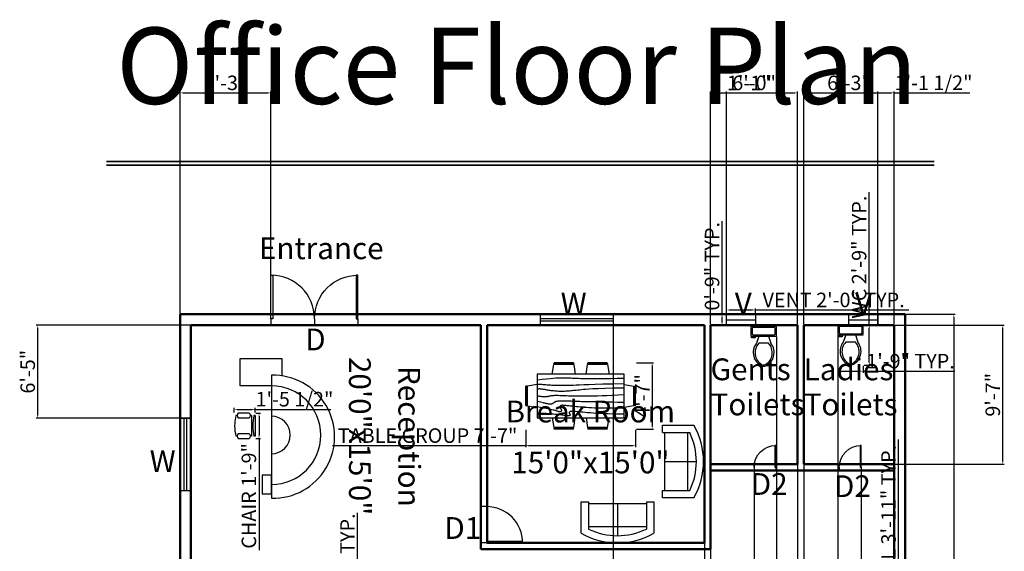
# Model space of a CAD drawing. Units: inches. Extents: x 1953 to 3378, y 1378 to 2530.
# Tile 4 of 5: x 1963 to 2778, y 2090 to 2530. Entities that reach past the tile are written whole.
import ezdxf

# ---------------------------------------------------------------- set-up
doc = ezdxf.new("R2010")
doc.units = ezdxf.units.IN
for name, color, linetype, lineweight in [('A-ANNO-DIMS', 2, 'Continuous', 18), ('A-ANNO-TEXT', 7, 'Continuous', 18), ('A-ANNO-TTLB', 7, 'Continuous', 35), ('A-AREA-IDEN', 4, 'Continuous', 18), ('A-DOOR', 4, 'Continuous', 25), ('A-FLOR-FIXT', 9, 'Continuous', 25), ('A-FURN', 50, 'Continuous', 25), ('wall', 7, 'Continuous', 50), ('windows', 180, 'Continuous', 25)]:
    doc.layers.add(name, color=color, linetype=linetype, lineweight=lineweight)
doc.styles.get("Standard").update_dxf_attribs({"font": 'arial.ttf'})
doc.dimstyles.new('ISO-25', dxfattribs={"dimtxt": 12, "dimasz": 2.5, "dimexe": 1.25, "dimexo": 0.625, "dimtad": 1, "dimdec": 1, "dimlunit": 4, "dimtxsty": 'Standard', "dimcen": 2.5, "dimadec": 0, "dimazin": 0, "dimtfac": 1, "dimtdec": 1, "dimtmove": 0, "dimatfit": 3, "dimfxl": 1, "dimarcsym": 0})

# ---------------------------------------------------------------- blocks, each defined once
blk = doc.blocks.new('*U7')
for p, q in [((0, 0), (0, -6)), ((-40, 0), (-40, -6))]:
    blk.add_line(p, q)
blk.add_lwpolyline([(0, 0), (0, 40), (-1.75, 40), (-1.75, 0)], close=True)
blk.add_arc((0, 0), 40, 90, 180)
blk = doc.blocks.new('*U2')
for p, q in [((0, 0), (0, -6)), ((40, 0), (40, -6))]:
    blk.add_line(p, q)
blk.add_lwpolyline([(0, 0), (0, 40), (1.75, 40), (1.75, 0)], close=True)
blk.add_arc((0, 0), 40, 0, 90)
blk = doc.blocks.new('Toilet - top')
for p, q in [((-8, -8.5), (-8, -8)), ((-7, -8), (-7, -9.5)), ((-4, -8), (-6, -14)), ((4, -8), (6, -14)), ((9.5, -6), (9.5, -2)), ((-10, -8.5), (-8, -8.5)), ((-10, -9.5), (-10, -8.5)), ((-7, -9.5), (-10, -9.5)), ((4, -14), (-4, -14))]:
    blk.add_line(p, q)
blk.add_lwpolyline([(10.5, -8), (10.5, 0), (-10.5, 0), (-10.5, -8)], close=True)
for points in [[(-9.5, -2), (-9.5, -6)], [(8.5, -1), (-8.5, -1)], [(-8.5, -7), (8.5, -7)]]:
    blk.add_lwpolyline(points)
for centre, radius, start, end in [((-8.62, -1.88), 0.884, 81.8699, 188.1301), ((-8.62, -6.12), 0.884, 171.8699, 278.1301), ((8.62, -1.88), 0.884, 351.8699, 98.1301), ((8.62, -6.12), 0.884, 261.8699, 8.1301), ((3.52, -21.58), 12.17, 141.46911, 247.97143), ((4.2, -21.82), 11.33, 136.36773, 238.94682), ((-3.52, -21.58), 12.17, 292.02843, 38.53071), ((-4.2, -21.82), 11.33, 301.05301, 43.63209), ((0, -27.88), 4, 245.73182, 294.26817), ((0, -29), 4, 254.86053, 285.13947)]:
    blk.add_arc(centre, radius, start, end)
blk = doc.blocks.new('Sofa - Roundback Loveseat 5 ft.')
for p, q in [((0, -32.44198), (0, -5.99998)), ((-24, -33.99998), (-24, -11.46958)), ((-23.9998, -13.38178), (23.99986, -13.38178)), ((24.00004, -33.99998), (24.00004, -11.46958)), ((-24, -32.44198), (24.00004, -32.44198))]:
    blk.add_line(p, q)
for points in [[(-24, -33.99998), (-30, -33.99998), (-30, -7.99998)], [(30.00004, -7.99998), (30.00004, -33.99998), (24.00004, -33.99998)]]:
    blk.add_lwpolyline(points)
for centre, radius, start, end in [((0, -60.24998), 60.24998, 60.13715, 119.8628), ((0, -61.38438), 55.38444, 64.32083, 115.6792)]:
    blk.add_arc(centre, radius, start, end)
blk = doc.blocks.new('Dining Set - 36 x 72 in.')
for p, q in [((-22.2343, 26.00059), (-23.4847, 17.99762)), ((-22.2304, 26), (-5.7608, 26)), ((-22, 27.5), (-22.1562, 26.50042)), ((-5.8416, 26.5), (-22.1534, 26.5)), ((-22, 27.5), (-6, 27.5)), ((-5.8437, 26.49966), (-6, 27.5)), ((-4.5152, 17.99762), (-5.7655, 25.99926)), ((5.7657, 26.00059), (4.5153, 17.99762)), ((5.7696, 26), (22.2392, 26)), ((6, 27.5), (5.8438, 26.50042)), ((22.1584, 26.5), (5.8466, 26.5)), ((6, 27.5), (22, 27.5)), ((22.1563, 26.49966), (22, 27.5)), ((23.4848, 17.99762), (22.2345, 25.99926)), ((36, 18), (-36, 18)), ((-36, 18), (-36, -18)), ((36, -18), (36, 18)), ((-45.5, 8), (-44.5004, 8.15617)), ((-44.5, -8.15843), (-44.5, 8.15338)), ((-44.0006, 8.23428), (-35.9976, 9.48474)), ((-44, 8.23041), (-44, -8.23915)), ((44.0006, 8.23428), (35.9976, 9.48474)), ((44, 8.23041), (44, -8.23915)), ((44.5, -8.15843), (44.5, 8.15338)), ((45.5, 8), (44.5005, 8.15617)), ((-45.5, 8), (-45.5, -8)), ((45.5, 8), (45.5, -8)), ((-44.4997, -8.15631), (-45.5, -8)), ((44.4997, -8.15631), (45.5, -8)), ((-35.9976, -9.48476), (-43.9993, -8.2345)), ((35.9976, -9.48476), (43.9993, -8.2345)), ((-36, -18), (36, -18)), ((-22.2343, -26.0006), (-23.4847, -17.99762)), ((-4.5152, -17.99762), (-5.7655, -25.99928)), ((5.7657, -26.0006), (4.5153, -17.99762)), ((23.4848, -17.99762), (22.2345, -25.99928)), ((-22.2304, -26), (-5.7608, -26)), ((-22, -27.5), (-22.1562, -26.50044)), ((-5.8416, -26.5), (-22.1534, -26.5)), ((-22, -27.5), (-6, -27.5)), ((-5.8437, -26.49967), (-6, -27.5)), ((5.7696, -26), (22.2392, -26)), ((6, -27.5), (5.8438, -26.50044)), ((22.1584, -26.5), (5.8466, -26.5)), ((6, -27.5), (22, -27.5)), ((22.1563, -26.49967), (22, -27.5))]:
    blk.add_line(p, q)
for points in [[(-36, 15), (-31.1772, 14.97754), (-26.8079, 14.91406), (-22.8538, 14.81543), (-19.276, 14.6875), (-16.0362, 14.53613), (-13.0957, 14.36718), (-10.4159, 14.18652), (-7.9583, 14), (-5.6904, 13.81315), (-3.6035, 13.63021), (-1.6954, 13.45508), (0.0365, 13.29166), (1.5945, 13.14388), (2.9811, 13.01562), (4.1988, 12.9108), (5.25, 12.83333), (6.1393, 12.78613), (6.8802, 12.76823), (7.4883, 12.77767), (7.9792, 12.8125), (8.3685, 12.87077), (8.6719, 12.95052), (8.9049, 13.0498), (9.0833, 13.16666), (9.2205, 13.29899), (9.3216, 13.44401), (9.3895, 13.59879), (9.4271, 13.76041), (9.4373, 13.92594), (9.4232, 14.09245), (9.3875, 14.257), (9.3333, 14.41666), (9.2638, 14.56917), (9.1836, 14.71484), (9.0975, 14.85465), (9.0104, 14.98958), (8.9272, 15.1206), (8.8529, 15.2487), (8.7922, 15.37483), (8.75, 15.5), (8.7305, 15.62467), (8.7344, 15.74739), (8.7617, 15.86621), (8.8125, 15.97916), (8.8867, 16.08431), (8.9844, 16.17968), (9.1055, 16.26334), (9.25, 16.33333), (9.4189, 16.38802), (9.6172, 16.42708), (9.8506, 16.45052), (10.125, 16.45833), (10.4463, 16.45052), (10.8203, 16.42708), (11.2529, 16.38802), (11.75, 16.33333), (12.3184, 16.26318), (12.9694, 16.17838), (13.7151, 16.07991), (14.5677, 15.96875), (15.5395, 15.84586), (16.6426, 15.71224), (17.8893, 15.56884), (19.2917, 15.41666), (20.859, 15.25667), (22.5879, 15.08984), (24.4721, 14.91715), (26.5052, 14.73958), (28.6809, 14.5581), (30.9929, 14.3737), (33.4347, 14.18733), (36, 14)], [(-36, 10), (-28.9766, 10.14274), (-23.1725, 10.20442), (-18.4241, 10.19775), (-14.5677, 10.13541), (-11.4399, 10.03011), (-8.877, 9.89453), (-6.7154, 9.74137), (-4.7917, 9.58333), (-2.9698, 9.43082), (-1.2246, 9.28515), (0.4415, 9.14534), (2.026, 9.01041), (3.5266, 8.87939), (4.9408, 8.7513), (6.266, 8.62516), (7.5, 8.5), (8.6411, 8.37549), (9.6914, 8.2539), (10.6538, 8.13818), (11.5312, 8.03125), (12.3267, 7.93603), (13.043, 7.85547), (13.6831, 7.79248), (14.25, 7.75), (14.7471, 7.7303), (15.1797, 7.73307), (15.5537, 7.75732), (15.875, 7.80208), (16.1494, 7.86637), (16.3828, 7.94922), (16.5811, 8.04964), (16.75, 8.16666), (16.8944, 8.29915), (17.0143, 8.44531), (17.1089, 8.60319), (17.1771, 8.77083), (17.218, 8.94629), (17.2305, 9.1276), (17.2137, 9.31282), (17.1667, 9.5), (17.0895, 9.6875), (16.987, 9.875), (16.8649, 10.0625), (16.7292, 10.25), (16.5856, 10.4375), (16.4401, 10.625), (16.2985, 10.8125), (16.1667, 11), (16.05, 11.18733), (15.9518, 11.3737), (15.8752, 11.5581), (15.8229, 11.73958), (15.798, 11.91715), (15.8034, 12.08984), (15.842, 12.25667), (15.9167, 12.41666), (16.0295, 12.56836), (16.1784, 12.70833), (16.3605, 12.83268), (16.5729, 12.9375), (16.8127, 13.01888), (17.0768, 13.07291), (17.3625, 13.0957), (17.6667, 13.08333), (17.9894, 13.03312), (18.3418, 12.94726), (18.7382, 12.82918), (19.1927, 12.68229), (19.7195, 12.51001), (20.3327, 12.31575), (21.0465, 12.10294), (21.875, 11.875), (22.8357, 11.63354), (23.959, 11.37304), (25.2786, 11.08618), (26.8282, 10.76562), (28.6414, 10.40405), (30.752, 9.99414), (33.1936, 9.52856), (36, 9)], [(-36, 5.5), (-30.7157, 5.3348), (-26.069, 5.20963), (-21.9946, 5.11767), (-18.4271, 5.05208), (-15.3009, 5.00602), (-12.5508, 4.97265), (-10.1112, 4.94515), (-7.9167, 4.91666), (-5.909, 4.88167), (-4.0586, 4.83984), (-2.3429, 4.79215), (-0.7396, 4.73958), (0.7739, 4.6831), (2.22, 4.6237), (3.6213, 4.56233), (5, 4.5), (6.373, 4.43782), (7.7344, 4.3776), (9.0723, 4.32129), (10.375, 4.27083), (11.6309, 4.22819), (12.8281, 4.19531), (13.9551, 4.17415), (15, 4.16666), (15.954, 4.17448), (16.819, 4.19791), (17.6001, 4.23698), (18.3021, 4.29166), (18.9299, 4.36198), (19.4883, 4.44791), (19.9823, 4.54948), (20.4167, 4.66666), (20.7969, 4.79899), (21.1302, 4.94401), (21.4245, 5.09879), (21.6875, 5.26041), (21.9271, 5.42594), (22.1511, 5.59245), (22.3672, 5.757), (22.5834, 5.91666), (22.8065, 6.06868), (23.0404, 6.21093), (23.2879, 6.34147), (23.5521, 6.45833), (23.8358, 6.55957), (24.142, 6.64323), (24.4735, 6.70735), (24.8334, 6.75), (25.2235, 6.76969), (25.642, 6.76692), (26.0858, 6.74267), (26.5521, 6.69791), (27.0379, 6.63362), (27.5404, 6.55078), (28.0565, 6.45036), (28.5834, 6.33333), (29.1242, 6.19987), (29.7071, 6.04687), (30.3661, 5.87044), (31.1354, 5.66666), (32.0493, 5.43164), (33.142, 5.16146), (34.4475, 4.85221), (36, 4.5)], [(-36, -1), (-30.7915, -0.6591), (-26.0195, -0.38216), (-21.6519, -0.16284), (-17.6563, 0.00521), (-14.0005, 0.12833), (-10.6523, 0.21289), (-7.5796, 0.26522), (-4.75, 0.29166), (-2.134, 0.29793), (0.2878, 0.28711), (2.5317, 0.26163), (4.6146, 0.22396), (6.5529, 0.17651), (8.3633, 0.12174), (10.0623, 0.06209), (11.6667, 0), (13.1899, -0.06201), (14.6341, -0.1211), (15.9982, -0.17432), (17.2813, -0.21875), (18.4823, -0.25147), (19.6003, -0.26953), (20.6343, -0.27002), (21.5834, -0.25), (22.4481, -0.20768), (23.2357, -0.14584), (23.9549, -0.06836), (24.6146, 0.02083), (25.2235, 0.11784), (25.7904, 0.21875), (26.3241, 0.31966), (26.8334, 0.41666), (27.3265, 0.50618), (27.8099, 0.58593), (28.2894, 0.65397), (28.7709, 0.70833), (29.2601, 0.74707), (29.763, 0.76823), (30.2855, 0.76985), (30.8334, 0.75), (31.4088, 0.70784), (31.9994, 0.64713), (32.589, 0.57275), (33.1615, 0.48958), (33.7008, 0.4025), (34.1908, 0.3164), (34.6153, 0.23616), (34.9584, 0.16666), (35.2099, 0.11165), (35.3848, 0.07031), (35.504, 0.04069), (35.5886, 0.02083), (35.6594, 0.00879), (35.7377, 0.0026), (35.8442, 0.00032), (36, 0)], [(-36, -6.5), (-27.1843, -6.31267), (-20.084, -6.1263), (-14.469, -5.9419), (-10.1094, -5.76042), (-6.7752, -5.58285), (-4.2363, -5.41016), (-2.2629, -5.24333), (-0.625, -5.08334), (0.8708, -4.93099), (2.2715, -4.78646), (3.5872, -4.64974), (4.8281, -4.52084), (6.0046, -4.39974), (7.127, -4.28646), (8.2053, -4.18099), (9.25, -4.08334), (10.2705, -3.99382), (11.2734, -3.91407), (12.2647, -3.84603), (13.25, -3.79167), (14.2354, -3.75293), (15.2266, -3.73177), (16.2295, -3.73015), (17.25, -3.75), (18.2912, -3.79248), (19.3451, -3.85547), (20.4009, -3.93604), (21.4479, -4.03125), (22.4754, -4.13819), (23.4727, -4.25391), (24.4289, -4.37549), (25.3334, -4.5), (26.1785, -4.62492), (26.9694, -4.74935), (27.7145, -4.87281), (28.4219, -4.99479), (29.1, -5.11483), (29.7572, -5.23242), (30.4016, -5.34709), (31.0417, -5.45834), (31.6837, -5.56437), (32.3262, -5.65821), (32.9658, -5.73153), (33.599, -5.77604), (34.2224, -5.78345), (34.8327, -5.74545), (35.4264, -5.65373), (36, -5.5)], [(-36, -10), (-26.4022, -9.81299), (-18.4675, -9.62891), (-11.9839, -9.45069), (-6.7396, -9.28125), (-2.5226, -9.12354), (0.8789, -8.98047), (3.6769, -8.85498), (6.0833, -8.75), (8.2767, -8.66765), (10.3021, -8.60677), (12.1712, -8.56543), (13.8958, -8.54167), (15.4876, -8.53353), (16.9583, -8.53907), (18.3197, -8.55632), (19.5834, -8.58334), (20.7616, -8.61841), (21.8685, -8.66081), (22.9188, -8.71004), (23.9271, -8.76563), (24.9081, -8.82707), (25.8763, -8.89388), (26.8465, -8.96558), (27.8334, -9.04167), (28.8474, -9.12118), (29.8828, -9.20117), (30.93, -9.27824), (31.9792, -9.34896), (33.0205, -9.40991), (34.0443, -9.45768), (35.0407, -9.48885), (36, -9.5)], [(-36, -14.5), (-30.0881, -14.33513), (-25.0332, -14.21224), (-20.7312, -14.12647), (-17.0781, -14.07292), (-13.97, -14.04671), (-11.3027, -14.04297), (-8.9724, -14.05681), (-6.875, -14.08334), (-4.9224, -14.11833), (-3.0905, -14.16016), (-1.3709, -14.20785), (0.2448, -14.26042), (1.7647, -14.3169), (3.1973, -14.3763), (4.5507, -14.43767), (5.8333, -14.5), (7.0554, -14.5621), (8.235, -14.62175), (9.3922, -14.67652), (10.5469, -14.72396), (11.7192, -14.76164), (12.929, -14.78711), (14.1965, -14.79794), (15.5417, -14.79167), (16.9933, -14.76424), (18.6152, -14.70508), (20.4804, -14.60197), (22.6615, -14.44271), (25.2312, -14.21509), (28.2624, -13.9069), (31.8277, -13.50594), (36, -13)]]:
    blk.add_lwpolyline(points)
blk = doc.blocks.new('Chair - Desk')
for p, q in [((-8.5, 0), (-8.5, -1)), ((-8.5, 0), (8.5, 0)), ((8.5, 0), (8.5, -1)), ((-10.5, -5), (-10.5, -14)), ((-8.5, -3), (-8.5, -4)), ((-8.5, -3), (8.5, -3)), ((-6.5, -14), (-6.5, -5)), ((-2, -3), (-2, -1.9355)), ((2, -1.9576), (2, -3)), ((6.5, -5), (6.5, -14)), ((8.5, -3), (8.5, -4)), ((10.5, -14), (10.5, -5)), ((-8.5, -15), (-8.5, -16)), ((8.5, -15), (8.5, -16))]:
    blk.add_line(p, q)
for centre, radius, start, end in [((-8.5, -6.5), 2.5, 36.8699, 143.1301), ((0, 34.625), 36.625, 256.5803, 283.4197), ((8.5, -6.5), 2.5, 36.8699, 143.1301), ((-8.5, -12.5), 2.5, 216.8699, 323.1301), ((0, 19.625), 36.625, 256.5803, 283.4197), ((8.5, -12.5), 2.5, 216.8699, 323.1301)]:
    blk.add_arc(centre, radius, start, end)
blk = doc.blocks.new('*D27')
at = {"layer": 'A-ANNO-DIMS', "color": 0, "lineweight": -2, "transparency": 16777216}
for p, q in [((2696.37, 2286.01), (2737.23, 2286.01)), ((2735.98, 2283.51), (2735.98, 1448.51)), ((2696.37, 1446.01), (2737.23, 1446.01))]:
    blk.add_line(p, q, dxfattribs=at)
at = {"layer": 'A-ANNO-DIMS', "color": 0, "transparency": 16777216}
for points in [[(2735.56, 2283.51), (2736.4, 2283.51), (2735.98, 2286.01)], [(2735.56, 1448.51), (2736.4, 1448.51), (2735.98, 1446.01)]]:
    blk.add_solid(points, dxfattribs=at)
at = {"layer": 'Defpoints', "color": 0, "transparency": 16777216}
for p in [(2695.75, 2286.01), (2695.75, 1446.01), (2735.98, 1446.01)]:
    blk.add_point(p, dxfattribs=at)
at = {"layer": 'A-ANNO-DIMS', "color": 0, "transparency": 16777216, "insert": (2729.23, 1866.01), "char_height": 12, "attachment_point": 5, "rotation": 90}
blk.add_mtext("70'", dxfattribs=at)
blk = doc.blocks.new('WINDOW-60IN')
for p, q in [((0, 5.5), (60, 5.5)), ((0, 5.5), (60, 5.5)), ((0, 3.5), (60, 3.5))]:
    blk.add_line(p, q)
blk.add_lwpolyline([(0, 9), (60, 9), (60, 0), (0, 0)], close=True)
blk = doc.blocks.new('VENT-24IN')
blk.add_line((0, 4.5), (24, 4.5))
blk.add_lwpolyline([(0, 9), (24, 9), (24, 0), (0, 0)], close=True)
blk = doc.blocks.new('DESK-SEMICIRCULAR')
blk.add_line((0.02, 7.63), (101.66, 7.63))
blk.add_lwpolyline([(82.57, 7.63), (82.57, 0), (98.08, 0), (98.08, 7.63)], close=True)
for centre, radius, start, end in [((50.84, 8.97), 50.84, 358.48644, 181.51356), ((49.55, 7.63), 40.78, 0, 180), ((49.41, 7.63), 15.51, 0, 180)]:
    blk.add_arc(centre, radius, start, end)
blk = doc.blocks.new('*D36')
at = {"layer": 'A-ANNO-DIMS', "color": 0, "lineweight": -2, "transparency": 16777216}
for p, q in [((2690.25, 2006.56), (2690.25, 2182.51)), ((2683.81, 2006.56), (2691.5, 2006.56)), ((2690.25, 1961.98), (2690.25, 2004.06)), ((2683.81, 1959.48), (2691.5, 1959.48))]:
    blk.add_line(p, q, dxfattribs=at)
at = {"layer": 'A-ANNO-DIMS', "color": 0, "transparency": 16777216}
for points in [[(2689.83, 2004.06), (2690.66, 2004.06), (2690.25, 2006.56)], [(2689.83, 1961.98), (2690.66, 1961.98), (2690.25, 1959.48)]]:
    blk.add_solid(points, dxfattribs=at)
at = {"layer": 'Defpoints', "color": 0, "transparency": 16777216}
for p in [(2683.18, 2006.56), (2690.25, 2006.56), (2683.18, 1959.48)]:
    blk.add_point(p, dxfattribs=at)
at = {"layer": 'A-ANNO-DIMS', "color": 0, "transparency": 16777216, "insert": (2683.49, 2095.79), "char_height": 12, "attachment_point": 5, "rotation": 90}
blk.add_mtext('TERMINAL 3\'-11" TYP.', dxfattribs=at)
blk = doc.blocks.new('*D43')
at = {"layer": 'A-ANNO-DIMS', "color": 0, "lineweight": -2, "transparency": 16777216}
for p, q in [((2242.73, 2017.01), (2242.73, 2121.86)), ((2230.75, 2017.01), (2243.98, 2017.01)), ((2242.73, 1982.84), (2242.73, 2014.51)), ((2230.75, 1980.34), (2243.98, 1980.34))]:
    blk.add_line(p, q, dxfattribs=at)
at = {"layer": 'A-ANNO-DIMS', "color": 0, "transparency": 16777216}
for points in [[(2242.31, 2014.51), (2243.14, 2014.51), (2242.73, 2017.01)], [(2242.31, 1982.84), (2243.14, 1982.84), (2242.73, 1980.34)]]:
    blk.add_solid(points, dxfattribs=at)
at = {"layer": 'Defpoints', "color": 0, "transparency": 16777216}
for p in [(2230.13, 2017.01), (2242.73, 2017.01), (2230.13, 1980.34)]:
    blk.add_point(p, dxfattribs=at)
at = {"layer": 'A-ANNO-DIMS', "color": 0, "transparency": 16777216, "insert": (2235.89, 2070.69), "char_height": 12, "attachment_point": 5, "rotation": 90}
blk.add_mtext('3\'-0 1/2" TYP.', dxfattribs=at)
blk = doc.blocks.new('*D52')
at = {"layer": 'A-ANNO-DIMS', "color": 0, "lineweight": -2, "transparency": 16777216}
for p, q in [((2381.74, 2190.4), (2381.74, 2176.12)), ((2472.74, 2190.4), (2472.74, 2176.12)), ((2381.74, 2177.37), (2221.89, 2177.37)), ((2470.24, 2177.37), (2384.24, 2177.37))]:
    blk.add_line(p, q, dxfattribs=at)
at = {"layer": 'A-ANNO-DIMS', "color": 0, "transparency": 16777216}
for points in [[(2384.24, 2177.79), (2384.24, 2176.95), (2381.74, 2177.37)], [(2470.24, 2177.79), (2470.24, 2176.95), (2472.74, 2177.37)]]:
    blk.add_solid(points, dxfattribs=at)
at = {"layer": 'Defpoints', "color": 0, "transparency": 16777216}
for p in [(2381.74, 2191.02), (2472.74, 2191.02), (2381.74, 2177.37)]:
    blk.add_point(p, dxfattribs=at)
at = {"layer": 'A-ANNO-DIMS', "color": 0, "transparency": 16777216, "insert": (2300.57, 2184.21), "char_height": 12, "attachment_point": 5}
blk.add_mtext('TABLE GROUP 7\'-7"', dxfattribs=at)
blk = doc.blocks.new('*D53')
at = {"layer": 'A-ANNO-DIMS', "color": 0, "lineweight": -2, "transparency": 16777216}
for p, q in [((2473.37, 2246.02), (2487.64, 2246.02)), ((2486.39, 2243.52), (2486.39, 2193.52)), ((2473.37, 2191.02), (2487.64, 2191.02))]:
    blk.add_line(p, q, dxfattribs=at)
at = {"layer": 'A-ANNO-DIMS', "color": 0, "transparency": 16777216}
for points in [[(2485.98, 2243.52), (2486.81, 2243.52), (2486.39, 2246.02)], [(2485.98, 2193.52), (2486.81, 2193.52), (2486.39, 2191.02)]]:
    blk.add_solid(points, dxfattribs=at)
at = {"layer": 'Defpoints', "color": 0, "transparency": 16777216}
for p in [(2472.74, 2246.02), (2472.74, 2191.02), (2486.39, 2191.02)]:
    blk.add_point(p, dxfattribs=at)
at = {"layer": 'A-ANNO-DIMS', "color": 0, "transparency": 16777216, "insert": (2479.77, 2218.52), "char_height": 12, "attachment_point": 5, "rotation": 90}
blk.add_mtext('4\'-7"', dxfattribs=at)
blk = doc.blocks.new('*D54')
at = {"layer": 'A-ANNO-DIMS', "color": 0, "lineweight": -2, "transparency": 16777216}
for p, q in [((2666.01, 2277), (2666.01, 2386.98)), ((2661.68, 2277), (2667.26, 2277)), ((2666.01, 2246.46), (2666.01, 2274.5)), ((2661.68, 2243.96), (2667.26, 2243.96))]:
    blk.add_line(p, q, dxfattribs=at)
at = {"layer": 'A-ANNO-DIMS', "color": 0, "transparency": 16777216}
for points in [[(2665.59, 2274.5), (2666.42, 2274.5), (2666.01, 2277)], [(2665.59, 2246.46), (2666.42, 2246.46), (2666.01, 2243.96)]]:
    blk.add_solid(points, dxfattribs=at)
at = {"layer": 'Defpoints', "color": 0, "transparency": 16777216}
for p in [(2661.05, 2277), (2666.01, 2277), (2661.05, 2243.96)]:
    blk.add_point(p, dxfattribs=at)
at = {"layer": 'A-ANNO-DIMS', "color": 0, "transparency": 16777216, "insert": (2659.18, 2333.24), "char_height": 12, "attachment_point": 5, "rotation": 90}
blk.add_mtext('WC 2\'-9" TYP.', dxfattribs=at)
blk = doc.blocks.new('*D55')
at = {"layer": 'A-ANNO-DIMS', "color": 0, "lineweight": -2, "transparency": 16777216}
for p, q in [((2640.05, 2243.33), (2640.05, 2237.75)), ((2661.05, 2243.33), (2661.05, 2237.75)), ((2642.55, 2239), (2658.55, 2239)), ((2661.05, 2239), (2736.82, 2239))]:
    blk.add_line(p, q, dxfattribs=at)
at = {"layer": 'A-ANNO-DIMS', "color": 0, "transparency": 16777216}
for points in [[(2642.55, 2239.42), (2642.55, 2238.58), (2640.05, 2239)], [(2658.55, 2239.42), (2658.55, 2238.58), (2661.05, 2239)]]:
    blk.add_solid(points, dxfattribs=at)
at = {"layer": 'Defpoints', "color": 0, "transparency": 16777216}
for p in [(2640.05, 2243.96), (2661.05, 2243.96), (2661.05, 2239)]:
    blk.add_point(p, dxfattribs=at)
at = {"layer": 'A-ANNO-DIMS', "color": 0, "transparency": 16777216, "insert": (2700.18, 2245.75), "char_height": 12, "attachment_point": 5}
blk.add_mtext('1\'-9" TYP.', dxfattribs=at)
blk = doc.blocks.new('*D56')
at = {"layer": 'A-ANNO-DIMS', "color": 0, "lineweight": -2, "transparency": 16777216}
for p, q in [((2547.85, 2286.64), (2547.85, 2290.86)), ((2550.35, 2289.61), (2569.35, 2289.61)), ((2571.85, 2286.64), (2571.85, 2290.86)), ((2571.85, 2289.61), (2698.73, 2289.61))]:
    blk.add_line(p, q, dxfattribs=at)
at = {"layer": 'A-ANNO-DIMS', "color": 0, "transparency": 16777216}
for points in [[(2550.35, 2290.03), (2550.35, 2289.19), (2547.85, 2289.61)], [(2569.35, 2290.03), (2569.35, 2289.19), (2571.85, 2289.61)]]:
    blk.add_solid(points, dxfattribs=at)
at = {"layer": 'Defpoints', "color": 0, "transparency": 16777216}
for p in [(2571.85, 2289.61), (2547.85, 2286.01), (2571.85, 2286.01)]:
    blk.add_point(p, dxfattribs=at)
at = {"layer": 'A-ANNO-DIMS', "color": 0, "transparency": 16777216, "insert": (2636.54, 2296.36), "char_height": 12, "attachment_point": 5}
blk.add_mtext('VENT 2\'-0" TYP.', dxfattribs=at)
blk = doc.blocks.new('*D57')
at = {"layer": 'A-ANNO-DIMS', "color": 0, "lineweight": -2, "transparency": 16777216}
for p, q in [((2544.25, 2286.01), (2544.25, 2362.91)), ((2547.22, 2286.01), (2543, 2286.01)), ((2544.25, 2279.51), (2544.25, 2283.51)), ((2547.22, 2277.01), (2543, 2277.01))]:
    blk.add_line(p, q, dxfattribs=at)
at = {"layer": 'A-ANNO-DIMS', "color": 0, "transparency": 16777216}
for points in [[(2543.83, 2283.51), (2544.67, 2283.51), (2544.25, 2286.01)], [(2543.83, 2279.51), (2544.67, 2279.51), (2544.25, 2277.01)]]:
    blk.add_solid(points, dxfattribs=at)
at = {"layer": 'Defpoints', "color": 0, "transparency": 16777216}
for p in [(2544.25, 2286.01), (2547.85, 2286.01), (2547.85, 2277.01)]:
    blk.add_point(p, dxfattribs=at)
at = {"layer": 'A-ANNO-DIMS', "color": 0, "transparency": 16777216, "insert": (2537.5, 2325.71), "char_height": 12, "attachment_point": 5, "rotation": 90}
blk.add_mtext('0\'-9" TYP.', dxfattribs=at)
blk = doc.blocks.new('*D58')
at = {"layer": 'A-ANNO-DIMS', "color": 0, "lineweight": -2, "transparency": 16777216}
for p, q in [((2158.58, 2204.32), (2162.35, 2204.32)), ((2161.1, 2201.82), (2161.1, 2185.82)), ((2158.58, 2183.32), (2162.35, 2183.32)), ((2161.1, 2183.32), (2161.1, 2091))]:
    blk.add_line(p, q, dxfattribs=at)
at = {"layer": 'A-ANNO-DIMS', "color": 0, "transparency": 16777216}
for points in [[(2160.68, 2201.82), (2161.52, 2201.82), (2161.1, 2204.32)], [(2160.68, 2185.82), (2161.52, 2185.82), (2161.1, 2183.32)]]:
    blk.add_solid(points, dxfattribs=at)
at = {"layer": 'Defpoints', "color": 0, "transparency": 16777216}
for p in [(2157.95, 2204.32), (2157.95, 2183.32), (2161.1, 2183.32)]:
    blk.add_point(p, dxfattribs=at)
at = {"layer": 'A-ANNO-DIMS', "color": 0, "transparency": 16777216, "insert": (2154.27, 2135.91), "char_height": 12, "attachment_point": 5, "rotation": 90}
blk.add_mtext('CHAIR 1\'-9"', dxfattribs=at)
blk = doc.blocks.new('*D59')
at = {"layer": 'A-ANNO-DIMS', "color": 0, "lineweight": -2, "transparency": 16777216}
for p, q in [((2140.62, 2204.95), (2140.62, 2208.72)), ((2157.95, 2204.95), (2157.95, 2208.72)), ((2143.12, 2207.47), (2155.45, 2207.47)), ((2157.95, 2207.47), (2220.43, 2207.47))]:
    blk.add_line(p, q, dxfattribs=at)
at = {"layer": 'A-ANNO-DIMS', "color": 0, "transparency": 16777216}
for points in [[(2143.12, 2207.89), (2143.12, 2207.06), (2140.62, 2207.47)], [(2155.45, 2207.89), (2155.45, 2207.06), (2157.95, 2207.47)]]:
    blk.add_solid(points, dxfattribs=at)
at = {"layer": 'Defpoints', "color": 0, "transparency": 16777216}
for p in [(2140.62, 2204.32), (2157.95, 2207.47), (2157.95, 2204.32)]:
    blk.add_point(p, dxfattribs=at)
at = {"layer": 'A-ANNO-DIMS', "color": 0, "transparency": 16777216, "insert": (2190.44, 2214.3), "char_height": 12, "attachment_point": 5}
blk.add_mtext('1\'-5 1/2"', dxfattribs=at)
blk = doc.blocks.new('*D60')
at = {"layer": 'A-ANNO-DIMS', "color": 0, "lineweight": -2, "transparency": 16777216}
for p, q in [((2534.75, 2277.64), (2534.75, 2470.27)), ((2537.25, 2469.02), (2604.25, 2469.02)), ((2606.75, 2277.64), (2606.75, 2470.27))]:
    blk.add_line(p, q, dxfattribs=at)
at = {"layer": 'A-ANNO-DIMS', "color": 0, "transparency": 16777216}
for points in [[(2537.25, 2469.44), (2537.25, 2468.61), (2534.75, 2469.02)], [(2604.25, 2469.44), (2604.25, 2468.61), (2606.75, 2469.02)]]:
    blk.add_solid(points, dxfattribs=at)
at = {"layer": 'Defpoints', "color": 0, "transparency": 16777216}
for p in [(2606.75, 2469.02), (2534.75, 2277.01), (2606.75, 2277.01)]:
    blk.add_point(p, dxfattribs=at)
at = {"layer": 'A-ANNO-DIMS', "color": 0, "transparency": 16777216, "insert": (2570.75, 2475.78), "char_height": 12, "attachment_point": 5}
blk.add_mtext('6\'-0"', dxfattribs=at)
blk = doc.blocks.new('*D61')
at = {"layer": 'A-ANNO-DIMS', "color": 0, "lineweight": -2, "transparency": 16777216}
for p, q in [((2611.75, 2277.64), (2611.75, 2470.27)), ((2614.25, 2469.02), (2684.25, 2469.02)), ((2686.75, 2277.64), (2686.75, 2470.27))]:
    blk.add_line(p, q, dxfattribs=at)
at = {"layer": 'A-ANNO-DIMS', "color": 0, "transparency": 16777216}
for points in [[(2614.25, 2469.44), (2614.25, 2468.61), (2611.75, 2469.02)], [(2684.25, 2469.44), (2684.25, 2468.61), (2686.75, 2469.02)]]:
    blk.add_solid(points, dxfattribs=at)
at = {"layer": 'Defpoints', "color": 0, "transparency": 16777216}
for p in [(2686.75, 2469.02), (2611.75, 2277.01), (2686.75, 2277.01)]:
    blk.add_point(p, dxfattribs=at)
at = {"layer": 'A-ANNO-DIMS', "color": 0, "transparency": 16777216, "insert": (2649.25, 2475.78), "char_height": 12, "attachment_point": 5}
blk.add_mtext('6\'-3"', dxfattribs=at)
blk = doc.blocks.new('*D62')
at = {"layer": 'A-ANNO-DIMS', "color": 0, "lineweight": -2, "transparency": 16777216}
for p, q in [((2687.37, 2277.01), (2777.76, 2277.01)), ((2776.51, 2164.51), (2776.51, 2274.51)), ((2687.37, 2162.01), (2777.76, 2162.01))]:
    blk.add_line(p, q, dxfattribs=at)
at = {"layer": 'A-ANNO-DIMS', "color": 0, "transparency": 16777216}
for points in [[(2776.09, 2274.51), (2776.93, 2274.51), (2776.51, 2277.01)], [(2776.09, 2164.51), (2776.93, 2164.51), (2776.51, 2162.01)]]:
    blk.add_solid(points, dxfattribs=at)
at = {"layer": 'Defpoints', "color": 0, "transparency": 16777216}
for p in [(2686.75, 2277.01), (2776.51, 2277.01), (2686.75, 2162.01)]:
    blk.add_point(p, dxfattribs=at)
at = {"layer": 'A-ANNO-DIMS', "color": 0, "transparency": 16777216, "insert": (2769.76, 2219.51), "char_height": 12, "attachment_point": 5, "rotation": 90}
blk.add_mtext('9\'-7"', dxfattribs=at)
blk = doc.blocks.new('*D63')
at = {"layer": 'A-ANNO-DIMS', "color": 0, "lineweight": -2, "transparency": 16777216}
for p, q in [((2095.75, 2286.64), (2095.75, 2470.27)), ((2098.25, 2469.02), (2168.5, 2469.02)), ((2171, 2283.04), (2171, 2470.27))]:
    blk.add_line(p, q, dxfattribs=at)
at = {"layer": 'A-ANNO-DIMS', "color": 0, "transparency": 16777216}
for points in [[(2098.25, 2469.44), (2098.25, 2468.61), (2095.75, 2469.02)], [(2168.5, 2469.44), (2168.5, 2468.61), (2171, 2469.02)]]:
    blk.add_solid(points, dxfattribs=at)
at = {"layer": 'Defpoints', "color": 0, "transparency": 16777216}
for p in [(2171, 2469.02), (2095.75, 2286.01), (2171, 2282.41)]:
    blk.add_point(p, dxfattribs=at)
at = {"layer": 'A-ANNO-DIMS', "color": 0, "transparency": 16777216, "insert": (2133.37, 2475.78), "char_height": 12, "attachment_point": 5}
blk.add_mtext('6\'-3"', dxfattribs=at)
blk = doc.blocks.new('*D69')
at = {"layer": 'A-ANNO-DIMS', "color": 0, "lineweight": -2, "transparency": 16777216}
for p, q in [((2104.12, 2277.01), (1976.77, 2277.01)), ((1978.02, 2202.63), (1978.02, 2274.51)), ((2104.12, 2200.13), (1976.77, 2200.13))]:
    blk.add_line(p, q, dxfattribs=at)
at = {"layer": 'A-ANNO-DIMS', "color": 0, "transparency": 16777216}
for points in [[(1977.6, 2274.51), (1978.44, 2274.51), (1978.02, 2277.01)], [(1977.6, 2202.63), (1978.44, 2202.63), (1978.02, 2200.13)]]:
    blk.add_solid(points, dxfattribs=at)
at = {"layer": 'Defpoints', "color": 0, "transparency": 16777216}
for p in [(1978.02, 2277.01), (2104.75, 2277.01), (2104.75, 2200.13)]:
    blk.add_point(p, dxfattribs=at)
at = {"layer": 'A-ANNO-DIMS', "color": 0, "transparency": 16777216, "insert": (1971.27, 2238.57), "char_height": 12, "attachment_point": 5, "rotation": 90}
blk.add_mtext('6\'-5"', dxfattribs=at)
blk = doc.blocks.new('*D74')
at = {"layer": 'A-ANNO-DIMS', "color": 0, "lineweight": -2, "transparency": 16777216}
for p, q in [((2454.07, 2276.39), (2454.07, 1387.78)), ((2529.75, 2276.39), (2529.75, 1387.78)), ((2456.57, 1389.03), (2527.25, 1389.03))]:
    blk.add_line(p, q, dxfattribs=at)
at = {"layer": 'A-ANNO-DIMS', "color": 0, "transparency": 16777216}
for points in [[(2456.57, 1389.45), (2456.57, 1388.62), (2454.07, 1389.03)], [(2527.25, 1389.45), (2527.25, 1388.62), (2529.75, 1389.03)]]:
    blk.add_solid(points, dxfattribs=at)
at = {"layer": 'Defpoints', "color": 0, "transparency": 16777216}
for p in [(2454.07, 2277.01), (2529.75, 2277.01), (2529.75, 1389.03)]:
    blk.add_point(p, dxfattribs=at)
at = {"layer": 'A-ANNO-DIMS', "color": 0, "transparency": 16777216, "insert": (2491.91, 1395.87), "char_height": 12, "attachment_point": 5}
blk.add_mtext('6\'-3 1/2"', dxfattribs=at)
blk = doc.blocks.new('*D78')
at = {"layer": 'A-ANNO-DIMS', "color": 0, "lineweight": -2, "transparency": 16777216}
for p, q in [((2534.75, 2277.64), (2534.75, 2470.27)), ((2537.25, 2469.02), (2545.35, 2469.02)), ((2547.85, 2277.64), (2547.85, 2470.27)), ((2547.85, 2469.02), (2582.37, 2469.02))]:
    blk.add_line(p, q, dxfattribs=at)
at = {"layer": 'A-ANNO-DIMS', "color": 0, "transparency": 16777216}
for points in [[(2537.25, 2469.44), (2537.25, 2468.61), (2534.75, 2469.02)], [(2545.35, 2469.44), (2545.35, 2468.61), (2547.85, 2469.02)]]:
    blk.add_solid(points, dxfattribs=at)
at = {"layer": 'Defpoints', "color": 0, "transparency": 16777216}
for p in [(2547.85, 2469.02), (2534.75, 2277.01), (2547.85, 2277.01)]:
    blk.add_point(p, dxfattribs=at)
at = {"layer": 'A-ANNO-DIMS', "color": 0, "transparency": 16777216, "insert": (2566.36, 2475.67), "char_height": 12, "attachment_point": 5}
blk.add_mtext('1\'-1"', dxfattribs=at)
blk = doc.blocks.new('*D79')
at = {"layer": 'A-ANNO-DIMS', "color": 0, "lineweight": -2, "transparency": 16777216}
for p, q in [((2673.25, 2277.64), (2673.25, 2470.27)), ((2675.75, 2469.02), (2684.25, 2469.02)), ((2686.75, 2277.64), (2686.75, 2470.27)), ((2686.75, 2469.02), (2749.23, 2469.02))]:
    blk.add_line(p, q, dxfattribs=at)
at = {"layer": 'A-ANNO-DIMS', "color": 0, "transparency": 16777216}
for points in [[(2675.75, 2469.44), (2675.75, 2468.61), (2673.25, 2469.02)], [(2684.25, 2469.44), (2684.25, 2468.61), (2686.75, 2469.02)]]:
    blk.add_solid(points, dxfattribs=at)
at = {"layer": 'Defpoints', "color": 0, "transparency": 16777216}
for p in [(2686.75, 2469.02), (2673.25, 2277.01), (2686.75, 2277.01)]:
    blk.add_point(p, dxfattribs=at)
at = {"layer": 'A-ANNO-DIMS', "color": 0, "transparency": 16777216, "insert": (2719.24, 2475.85), "char_height": 12, "attachment_point": 5}
blk.add_mtext('1\'-1 1/2"', dxfattribs=at)
blk = doc.blocks.new('*D80')
at = {"layer": 'A-ANNO-DIMS', "color": 0, "lineweight": -2, "transparency": 16777216}
for p, q in [((2534.75, 2161.39), (2534.75, 1387.78)), ((2570.9, 2161.44), (2570.9, 1387.78)), ((2537.25, 1389.03), (2568.4, 1389.03))]:
    blk.add_line(p, q, dxfattribs=at)
at = {"layer": 'A-ANNO-DIMS', "color": 0, "transparency": 16777216}
for points in [[(2537.25, 1389.45), (2537.25, 1388.62), (2534.75, 1389.03)], [(2568.4, 1389.45), (2568.4, 1388.62), (2570.9, 1389.03)]]:
    blk.add_solid(points, dxfattribs=at)
at = {"layer": 'Defpoints', "color": 0, "transparency": 16777216}
for p in [(2534.75, 2162.01), (2570.9, 2162.07), (2570.9, 1389.03)]:
    blk.add_point(p, dxfattribs=at)
at = {"layer": 'A-ANNO-DIMS', "color": 0, "transparency": 16777216, "insert": (2552.82, 1395.79), "char_height": 12, "attachment_point": 5}
blk.add_mtext('3\'-0"', dxfattribs=at)
blk = doc.blocks.new('*D81')
at = {"layer": 'A-ANNO-DIMS', "color": 0, "lineweight": -2, "transparency": 16777216}
for p, q in [((2659.25, 2159.09), (2659.25, 1387.78)), ((2686.75, 2161.39), (2686.75, 1387.78)), ((2661.75, 1389.03), (2684.25, 1389.03)), ((2686.75, 1389.03), (2750.56, 1389.03))]:
    blk.add_line(p, q, dxfattribs=at)
at = {"layer": 'A-ANNO-DIMS', "color": 0, "transparency": 16777216}
for points in [[(2661.75, 1389.45), (2661.75, 1388.62), (2659.25, 1389.03)], [(2684.25, 1389.45), (2684.25, 1388.62), (2686.75, 1389.03)]]:
    blk.add_solid(points, dxfattribs=at)
at = {"layer": 'Defpoints', "color": 0, "transparency": 16777216}
for p in [(2659.25, 2159.71), (2686.75, 2162.01), (2686.75, 1389.03)]:
    blk.add_point(p, dxfattribs=at)
at = {"layer": 'A-ANNO-DIMS', "color": 0, "transparency": 16777216, "insert": (2719.91, 1395.87), "char_height": 12, "attachment_point": 5}
blk.add_mtext('2\'-3 1/2"', dxfattribs=at)
blk = doc.blocks.new('*D82')
at = {"layer": 'A-ANNO-DIMS', "color": 0, "lineweight": -2, "transparency": 16777216}
for p, q in [((2606.75, 2161.39), (2606.75, 1387.78)), ((2611.75, 2161.39), (2611.75, 1387.78)), ((2604.25, 1389.03), (2601.75, 1389.03)), ((2606.75, 1389.03), (2611.75, 1389.03)), ((2614.25, 1389.03), (2649.9, 1389.03))]:
    blk.add_line(p, q, dxfattribs=at)
at = {"layer": 'A-ANNO-DIMS', "color": 0, "transparency": 16777216}
for points in [[(2604.25, 1389.45), (2604.25, 1388.62), (2606.75, 1389.03)], [(2614.25, 1389.45), (2614.25, 1388.62), (2611.75, 1389.03)]]:
    blk.add_solid(points, dxfattribs=at)
at = {"layer": 'Defpoints', "color": 0, "transparency": 16777216}
for p in [(2606.75, 2162.01), (2611.75, 2162.01), (2611.75, 1389.03)]:
    blk.add_point(p, dxfattribs=at)
at = {"layer": 'A-ANNO-DIMS', "color": 0, "transparency": 16777216, "insert": (2633.32, 1395.79), "char_height": 12, "attachment_point": 5}
blk.add_mtext('0\'-5"', dxfattribs=at)
blk = doc.blocks.new('*D84')
at = {"layer": 'A-ANNO-DIMS', "color": 0, "lineweight": -2, "transparency": 16777216}
for p, q in [((2606.75, 2276.39), (2606.75, 1387.78)), ((2589.14, 2267.41), (2589.14, 1387.78)), ((2591.64, 1389.03), (2604.25, 1389.03)), ((2606.75, 1389.03), (2669.23, 1389.03))]:
    blk.add_line(p, q, dxfattribs=at)
at = {"layer": 'A-ANNO-DIMS', "color": 0, "transparency": 16777216}
for points in [[(2591.64, 1389.45), (2591.64, 1388.62), (2589.14, 1389.03)], [(2604.25, 1389.45), (2604.25, 1388.62), (2606.75, 1389.03)]]:
    blk.add_solid(points, dxfattribs=at)
at = {"layer": 'Defpoints', "color": 0, "transparency": 16777216}
for p in [(2606.75, 2277.01), (2589.14, 2268.03), (2606.75, 1389.03)]:
    blk.add_point(p, dxfattribs=at)
at = {"layer": 'A-ANNO-DIMS', "color": 0, "transparency": 16777216, "insert": (2639.24, 1395.86), "char_height": 12, "attachment_point": 5}
blk.add_mtext('1\'-5 1/2"', dxfattribs=at)
blk = doc.blocks.new('*D85')
at = {"layer": 'A-ANNO-DIMS', "color": 0, "lineweight": -2, "transparency": 16777216}
for p, q in [((2611.75, 2276.39), (2611.75, 1387.78)), ((2640.05, 2268.38), (2640.05, 1387.78)), ((2614.25, 1389.03), (2637.55, 1389.03)), ((2640.05, 1389.03), (2703.87, 1389.03))]:
    blk.add_line(p, q, dxfattribs=at)
at = {"layer": 'A-ANNO-DIMS', "color": 0, "transparency": 16777216}
for points in [[(2614.25, 1389.45), (2614.25, 1388.62), (2611.75, 1389.03)], [(2637.55, 1389.45), (2637.55, 1388.62), (2640.05, 1389.03)]]:
    blk.add_solid(points, dxfattribs=at)
at = {"layer": 'Defpoints', "color": 0, "transparency": 16777216}
for p in [(2611.75, 2277.01), (2640.05, 2269), (2640.05, 1389.03)]:
    blk.add_point(p, dxfattribs=at)
at = {"layer": 'A-ANNO-DIMS', "color": 0, "transparency": 16777216, "insert": (2673.21, 1395.86), "char_height": 12, "attachment_point": 5}
blk.add_mtext('2\'-4 1/2"', dxfattribs=at)

msp = doc.modelspace()

# ---------------------------------------------------------------- linework, layer by layer
at = {"layer": 'A-ANNO-TTLB'}
for p, q in [((2034.82, 2412.22), (2719.71, 2412.22)), ((2034.82, 2409.22), (2719.71, 2409.22))]:
    msp.add_line(p, q, dxfattribs=at)
at = {"layer": 'A-FURN'}
msp.add_lwpolyline([(2171.47, 2226.88), (2145.48, 2226.88), (2145.48, 2249.4), (2179.99, 2249.4), (2179.99, 2235.15)], dxfattribs=at)
at = {"layer": 'wall'}
for p, q in [((2095.75, 2286.01), (2695.75, 2286.01)), ((2095.75, 1446.01), (2095.75, 2286.01)), ((2695.75, 2286.01), (2695.75, 1446.01)), ((2104.75, 2277.01), (2344.75, 2277.01)), ((2104.75, 2020.01), (2104.75, 2277.01)), ((2344.75, 2092.01), (2344.75, 2277.01)), ((2349.75, 2097.01), (2349.75, 2277.01)), ((2349.75, 2277.01), (2529.75, 2277.01)), ((2529.75, 2097.01), (2529.75, 2277.01)), ((2534.75, 2092.01), (2534.75, 2277.01)), ((2534.75, 2277.01), (2606.75, 2277.01)), ((2606.75, 2162.01), (2606.75, 2277.01)), ((2611.75, 2162.01), (2611.75, 2277.01)), ((2611.75, 2277.01), (2686.75, 2277.01)), ((2686.75, 2277.01), (2686.75, 2097.01)), ((2534.75, 2162.01), (2606.75, 2162.01)), ((2611.75, 2162.01), (2686.75, 2162.01)), ((2534.75, 2157.01), (2606.75, 2157.01)), ((2606.75, 2157.01), (2686.75, 2157.01)), ((2686.75, 2157.01), (2686.75, 2011)), ((2349.75, 2097.01), (2529.75, 2097.01)), ((2344.75, 2092.01), (2534.75, 2092.01))]:
    msp.add_line(p, q, dxfattribs=at)

# ---------------------------------------------------------------- block references
at = {"layer": 'A-DOOR'}
for p, xscale, yscale, zscale in [((2171, 2282.41), 0.9, 0.9, 0.9), ((2243, 2282.41), -0.9, 0.9, 0.9), ((2588.75, 2159.71), -0.45, 0.45, 0.45), ((2659.25, 2159.71), -0.45, 0.45, 0.45)]:
    msp.add_blockref('*U2', p, dxfattribs=dict(at, xscale=xscale, yscale=yscale, zscale=zscale))
at = {"layer": 'A-DOOR', "xscale": 0.75, "yscale": 0.75, "zscale": 0.75, "rotation": 270}
msp.add_blockref('*U7', (2349.25, 2097.04), dxfattribs=at)
at = {"layer": 'A-FLOR-FIXT'}
for p in [(2578.64, 2276.03), (2650.55, 2277)]:
    msp.add_blockref('Toilet - top', p, dxfattribs=at)
at = {"layer": 'A-FURN'}
for name, p, rotation in [('Dining Set - 36 x 72 in.', (2427.24, 2218.52), 180), ('DESK-SEMICIRCULAR', (2163.84, 2235.65), 270.0000000000197), ('Chair - Desk', (2157.95, 2193.82), 270), ('Sofa - Roundback Loveseat 5 ft.', (2528.95, 2164.25), 270), ('Sofa - Roundback Loveseat 5 ft.', (2457.68, 2097.01), 180)]:
    msp.add_blockref(name, p, dxfattribs=dict(at, rotation=rotation))
at = {"layer": 'windows'}
for name, p in [('WINDOW-60IN', (2394.07, 2277.01)), ('VENT-24IN', (2547.85, 2277.01)), ('VENT-24IN', (2649.25, 2277.01))]:
    msp.add_blockref(name, p, dxfattribs=at)
at = {"layer": 'windows', "rotation": 90.00000000000078}
msp.add_blockref('WINDOW-60IN', (2104.75, 2140.13), dxfattribs=at)

# ---------------------------------------------------------------- texts
at = {"layer": 'A-ANNO-TEXT'}
for s, p in [('W', (2410.67, 2286.01)), ('V', (2554.72, 2286.01)), ('V', (2654.27, 2286.01)), ('D', (2199.33, 2256.25)), ('W', (2070.61, 2155.68)), ('D2', (2567.97, 2136.74)), ('D2', (2636.8, 2134.92)), ('D1', (2314.43, 2100.36))]:
    msp.add_text(s, height=18, dxfattribs=at).set_placement(p)
at = {"layer": 'A-ANNO-TTLB'}
msp.add_text('Office Floor Plan', height=63.0672, dxfattribs=at).set_placement((2042.98, 2459.92))
at = {"layer": 'A-AREA-IDEN'}
for s, p in [('Entrance', (2161.01, 2331.6)), ('Gents', (2534.75, 2231.53)), ('Ladies', (2611.75, 2231.52)), ('Break Room', (2365.07, 2196.69)), ('Toilets', (2534.75, 2202.55)), ('Toilets', (2611.75, 2202.55)), ('15\'0"x15\'0"', (2369.82, 2154.54))]:
    msp.add_text(s, height=18, dxfattribs=at).set_placement(p)
for s, p in [('20\'0"x15\'0"', (2235.55, 2250.81)), ('Reception', (2276.43, 2243.36))]:
    msp.add_text(s, height=18, rotation=270, dxfattribs=at).set_placement(p)

# ---------------------------------------------------------------- dimensions: what is measured, and where the dimension line sits
at = {"layer": 'A-ANNO-DIMS'}
for base, p1, p2, picture, middle in [((2686.75, 2469.02), (2673.25, 2277.01), (2686.75, 2277.01), '*D79', (2719.24, 2475.85)), ((2170.9966, 2469.0246), (2095.7476, 2286.0108), (2170.9966, 2282.4108), '*D63', (2133.3721, 2475.7806)), ((2606.75, 2469.02), (2534.75, 2277.01), (2606.75, 2277.01), '*D60', (2570.75, 2475.78)), ((2547.85, 2469.02), (2534.75, 2277.01), (2547.85, 2277.01), '*D78', (2566.36, 2475.67)), ((2686.75, 2469.02), (2611.75, 2277.01), (2686.75, 2277.01), '*D61', (2649.25, 2475.78)), ((2529.75, 1389.03), (2454.07, 2277.01), (2529.75, 2277.01), '*D74', (2491.91, 1395.87)), ((2606.75, 1389.03), (2589.14, 2268.03), (2606.75, 2277.01), '*D84', (2639.24, 1395.86)), ((2640.05, 1389.03), (2611.75, 2277.01), (2640.05, 2269), '*D85', (2673.21, 1395.86)), ((2157.95, 2207.47), (2140.62, 2204.32), (2157.95, 2204.32), '*D59', (2190.44, 2214.3)), ((2570.9022, 1389.0336), (2534.7476, 2162.0108), (2570.9022, 2162.0653), '*D80', (2552.8249, 1395.7895)), ((2611.75, 1389.03), (2606.75, 2162.01), (2611.75, 2162.01), '*D82', (2633.32, 1395.79)), ((2686.75, 1389.03), (2659.25, 2159.71), (2686.75, 2162.01), '*D81', (2719.91, 1395.87))]:
    dim = msp.add_linear_dim(base=base, p1=p1, p2=p2, dimstyle='ISO-25', override={"dimdec": 1, "dimlfac": 1, "dimrnd": 0, "dimzin": 1, "dimdsep": 46, "dimlunit": 4, "dimfrac": 2}, dxfattribs=at)
    dim.commit()
    dim.dimension.update_dxf_attribs({"geometry": picture, "text_midpoint": middle})
for base, p1, p2, angle, text, picture, middle in [((2666.01, 2277), (2661.05, 2243.96), (2661.05, 2277), 90, 'WC <> TYP.', '*D54', (2659.18, 2333.24)), ((2544.25, 2286.01), (2547.85, 2277.01), (2547.85, 2286.01), 90, '<> TYP.', '*D57', (2537.5, 2325.71)), ((2381.74, 2177.37), (2472.74, 2191.02), (2381.74, 2191.02), 180, 'TABLE GROUP <>', '*D52', (2300.57, 2184.21)), ((2161.1, 2183.32), (2157.95, 2204.32), (2157.95, 2183.32), 270, 'CHAIR <>', '*D58', (2154.27, 2135.91)), ((2690.25, 2006.56), (2683.18, 1959.48), (2683.18, 2006.56), 90, 'TERMINAL <> TYP.', '*D36', (2683.49, 2095.79)), ((2242.73, 2017.01), (2230.13, 1980.34), (2230.13, 2017.01), 90, '<> TYP.', '*D43', (2235.89, 2070.69))]:
    dim = msp.add_linear_dim(base=base, p1=p1, p2=p2, angle=angle, text=text, dimstyle='ISO-25', override={"dimdec": 1, "dimlfac": 1, "dimrnd": 0, "dimzin": 1, "dimdsep": 46, "dimlunit": 4, "dimfrac": 2}, dxfattribs=at)
    dim.commit()
    dim.dimension.update_dxf_attribs({"geometry": picture, "text_midpoint": middle})
for base, p1, p2, text, picture, middle in [((2571.85, 2289.61), (2547.85, 2286.01), (2571.85, 2286.01), 'VENT <> TYP.', '*D56', (2636.54, 2296.36)), ((2661.05, 2239), (2640.05, 2243.96), (2661.05, 2243.96), '<> TYP.', '*D55', (2700.18, 2245.75))]:
    dim = msp.add_linear_dim(base=base, p1=p1, p2=p2, text=text, dimstyle='ISO-25', override={"dimdec": 1, "dimlfac": 1, "dimrnd": 0, "dimzin": 1, "dimdsep": 46, "dimlunit": 4, "dimfrac": 2}, dxfattribs=at)
    dim.commit()
    dim.dimension.update_dxf_attribs({"geometry": picture, "text_midpoint": middle})
for base, p1, p2, angle, override, picture, middle in [((2735.98, 1446.01), (2695.75, 2286.01), (2695.75, 1446.01), 90, {"dimclrd": 0, "dimclre": 0, "dimclrt": 0}, '*D27', (2729.23, 1866.01)), ((1978.02, 2277.01), (2104.75, 2200.13), (2104.75, 2277.01), 90, {"dimdec": 1, "dimlfac": 1, "dimrnd": 0, "dimzin": 1, "dimdsep": 46, "dimlunit": 4, "dimfrac": 2}, '*D69', (1971.27, 2238.57)), ((2776.51, 2277.01), (2686.75, 2162.01), (2686.75, 2277.01), 90, {"dimdec": 1, "dimlfac": 1, "dimrnd": 0, "dimzin": 1, "dimdsep": 46, "dimlunit": 4, "dimfrac": 2}, '*D62', (2769.76, 2219.51)), ((2486.39, 2191.02), (2472.74, 2246.02), (2472.74, 2191.02), 270, {"dimdec": 1, "dimlfac": 1, "dimrnd": 0, "dimzin": 1, "dimdsep": 46, "dimlunit": 4, "dimfrac": 2}, '*D53', (2479.77, 2218.52))]:
    dim = msp.add_linear_dim(base=base, p1=p1, p2=p2, angle=angle, dimstyle='ISO-25', override=override, dxfattribs=at)
    dim.commit()
    dim.dimension.update_dxf_attribs({"geometry": picture, "text_midpoint": middle})

doc.saveas('drawing.dxf')
